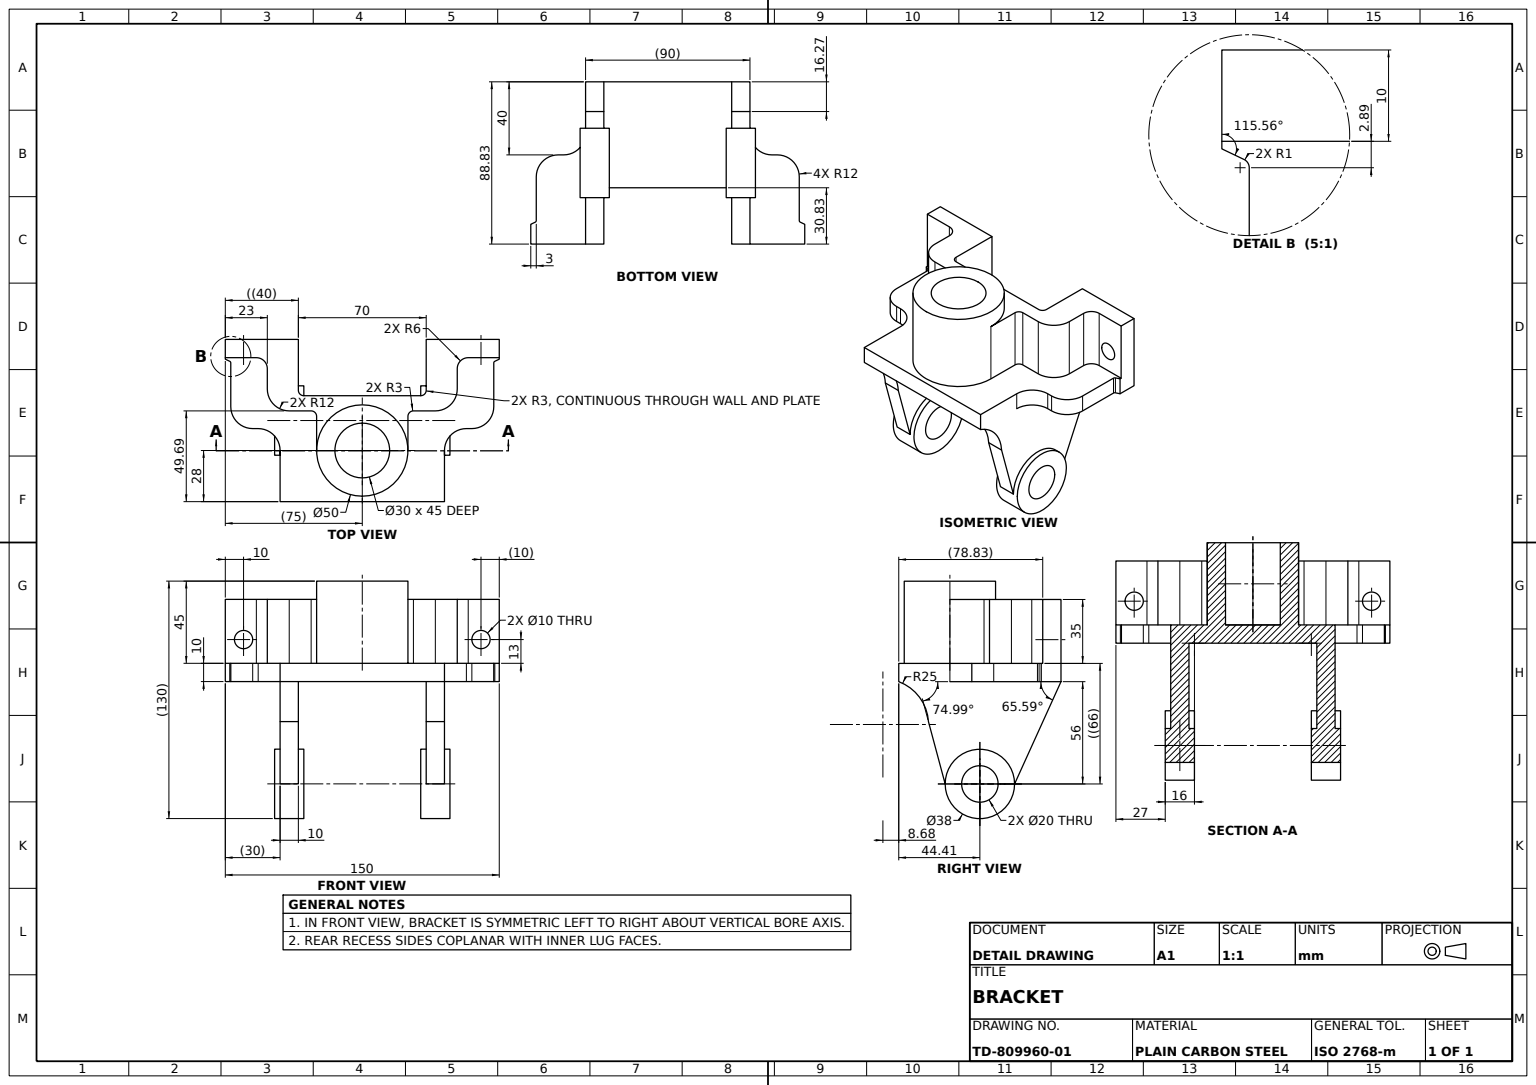
from build123d import *

# Parameters (mm, degrees)
BASE_PLATE_DEPTH        = 5
RISER_BLOCK_SKETCH_W    = 40
RISER_BLOCK_SKETCH_H    = 10.827146282
RISER_BLOCK_DEPTH       = 10
UPRIGHT_START           = 35
UPRIGHT_BOSS_35MM_DEPTH = 35
UPRIGHT_START_2         = 45
UPRIGHT_BOSS_45MM_DEPTH = 45
BORE_SKETCH_R           = 5
BORE_CUT_DEPTH          = 22.5
MOUNTING_LUG_DEPTH      = 10
LUG_BOSS_SKETCH_R       = 19
LUG_BOSS_SKETCH_R_2     = 10
LUG_BOSS_DEPTH          = 8


with BuildPart() as part:
    # Base Plate Sketch → Base Plate (new, symmetric)
    with BuildSketch(Plane(origin=(0, 0, 0), x_dir=(1, 0, 0), z_dir=(0, 1, 0))):
        with BuildLine():
            Line((-45, 0), (45, 0))
            Line((45, 0), (45, 28))
            ThreePointArc((45, 28), (48.514718626, 36.485281374), (57, 40))
            Line((57, 40), (60, 40))
            ThreePointArc((60, 40), (68.485281374, 43.514718626), (72, 52))
            Line((72, 52), (72, 75.935046753))
            ThreePointArc((72, 75.935046753), (72.153997607, 76.468225851), (72.568559901, 76.837188339))
            Line((72.568559901, 76.837188339), (75, 78))
            Line((75, 78), (72, 78))
            Line((72, 78), (35, 78))
            Line((35, 78), (35, 61))
            ThreePointArc((35, 61), (34.121320344, 58.878679656), (32, 58))
            Line((32, 58), (-32, 58))
            ThreePointArc((-32, 58), (-34.121320344, 58.878679656), (-35, 61))
            Line((-35, 61), (-35, 78))
            Line((-35, 78), (-72, 78))
            Line((-72, 78), (-75, 78))
            Line((-75, 78), (-72.568559901, 76.837188339))
            ThreePointArc((-72.568559901, 76.837188339), (-72.153997607, 76.468225851), (-72, 75.935046753))
            Line((-72, 75.935046753), (-72, 52))
            ThreePointArc((-72, 52), (-68.485281374, 43.514718626), (-60, 40))
            Line((-60, 40), (-57, 40))
            ThreePointArc((-57, 40), (-48.514718626, 36.485281374), (-45, 28))
            Line((-45, 28), (-45, 0))
        make_face()
    extrude(amount=BASE_PLATE_DEPTH, both=True)

    # Riser Block Sketch → Riser Block (add)
    with BuildSketch(Plane(origin=(0, 5, 0), x_dir=(1, 0, 0), z_dir=(0, 1, 0))):
        with Locations((-55, 83.413573141)):
            Rectangle(RISER_BLOCK_SKETCH_W, RISER_BLOCK_SKETCH_H)
        with Locations((55, 83.413573141)):
            Rectangle(RISER_BLOCK_SKETCH_W, RISER_BLOCK_SKETCH_H)
    extrude(amount=-RISER_BLOCK_DEPTH)

    # Upright Bosses Sketch → Upright Boss 35mm (add)
    with BuildSketch(Plane(origin=(0, 5, 0), x_dir=(1, 0, 0), z_dir=(0, 1, 0)).offset(UPRIGHT_START)):
        with BuildLine():
            Line((0, 53), (0, 58))
            Line((0, 58), (-32, 58))
            ThreePointArc((-32, 58), (-34.121320344, 58.878679656), (-35, 61))
            Line((-35, 61), (-35, 88.827146282))
            Line((-35, 88.827146282), (-75, 88.827146282))
            Line((-75, 88.827146282), (-75, 78.827146282))
            Line((-75, 78.827146282), (-58, 78.827146282))
            ThreePointArc((-58, 78.827146282), (-53.757359313, 77.069786969), (-52, 72.827146282))
            Line((-52, 72.827146282), (-52, 61.686127822))
            ThreePointArc((-52, 61.686127822), (-48.485281374, 53.200846447), (-40, 49.686127822))
            Line((-40, 49.686127822), (-28, 49.686127822))
            ThreePointArc((-28, 49.686127822), (-25.878679656, 48.807448165), (-25, 46.686127822))
            Line((-25, 46.686127822), (-25, 28))
            ThreePointArc((-25, 28), (-17.67766953, 45.67766953), (0, 53))
        make_face()
        with BuildLine():
            Line((75, 78.827146282), (75, 88.827146282))
            Line((75, 88.827146282), (35, 88.827146282))
            Line((35, 88.827146282), (35, 61))
            ThreePointArc((35, 61), (34.121320344, 58.878679656), (32, 58))
            Line((32, 58), (0, 58))
            Line((0, 58), (0, 53))
            ThreePointArc((0, 53), (17.67766953, 45.67766953), (25, 28))
            Line((25, 28), (25, 46.686127822))
            ThreePointArc((25, 46.686127822), (25.878679656, 48.807448165), (28, 49.686127822))
            Line((28, 49.686127822), (40, 49.686127822))
            ThreePointArc((40, 49.686127822), (48.485281374, 53.200846447), (52, 61.686127822))
            Line((52, 61.686127822), (52, 72.827146282))
            ThreePointArc((52, 72.827146282), (53.757359313, 77.069786969), (58, 78.827146282))
            Line((58, 78.827146282), (75, 78.827146282))
        make_face()
    extrude(amount=-UPRIGHT_BOSS_35MM_DEPTH)

    # Sketch5_3 → Upright Boss 45mm (add)
    with BuildSketch(Plane(origin=(0, 5, 0), x_dir=(1, 0, 0), z_dir=(0, 1, 0)).offset(UPRIGHT_START_2)):
        with BuildLine():
            ThreePointArc((25, 28), (17.67766953, 45.67766953), (0, 53))
            Line((0, 53), (0, 43))
            ThreePointArc((0, 43), (10.606601718, 38.606601718), (15, 28))
            ThreePointArc((15, 28), (10.606601718, 17.393398282), (0, 13))
            Line((0, 13), (0, 3))
            ThreePointArc((0, 3), (17.67766953, 10.32233047), (25, 28))
        make_face()
        with BuildLine():
            Line((0, 43), (0, 53))
            ThreePointArc((0, 53), (-17.67766953, 45.67766953), (-25, 28))
            ThreePointArc((-25, 28), (-17.67766953, 10.32233047), (0, 3))
            Line((0, 3), (0, 13))
            ThreePointArc((0, 13), (-15, 28), (0, 43))
        make_face()
        with BuildLine():
            ThreePointArc((25, 28), (17.67766953, 45.67766953), (0, 53))
            Line((0, 53), (0, 43))
            ThreePointArc((0, 43), (10.606601718, 38.606601718), (15, 28))
            ThreePointArc((15, 28), (10.606601718, 17.393398282), (0, 13))
            Line((0, 13), (0, 3))
            ThreePointArc((0, 3), (17.67766953, 10.32233047), (25, 28))
        make_face()
        with BuildLine():
            Line((0, 43), (0, 53))
            ThreePointArc((0, 53), (-17.67766953, 45.67766953), (-25, 28))
            ThreePointArc((-25, 28), (-17.67766953, 10.32233047), (0, 3))
            Line((0, 3), (0, 13))
            ThreePointArc((0, 13), (-15, 28), (0, 43))
        make_face()
    extrude(amount=-UPRIGHT_BOSS_45MM_DEPTH)

    # Bore Sketch → Bore Cut (cut, symmetric)
    with BuildSketch(Plane(origin=(0, 0, -88.827146282), x_dir=(-1, 0, 0), z_dir=(0, 0, -1))):
        with Locations((65, 18)):
            Circle(BORE_SKETCH_R)
        with Locations((-65, 18)):
            Circle(BORE_SKETCH_R)
    extrude(amount=BORE_CUT_DEPTH, both=True, mode=Mode.SUBTRACT)

    # Mounting Lug Sketch → Mounting Lug (add)
    with BuildSketch(Plane.ZY.offset(45)):
        with BuildLine():
            Line((-44.413573141, -5), (-88.827146282, -5))
            Line((-88.827146282, -5), (-63.413573141, -61))
            ThreePointArc((-63.413573141, -61), (-57.848601984, -47.564971157), (-44.413573141, -42))
            Line((-44.413573141, -42), (-44.413573141, -5))
        make_face()
        with BuildLine():
            Line((-28, -5), (-44.413573141, -5))
            Line((-44.413573141, -5), (-44.413573141, -42))
            ThreePointArc((-44.413573141, -42), (-30.978544299, -47.564971157), (-25.413573141, -61))
            Line((-25.413573141, -61), (-16.270280631, -26.90885398))
            ThreePointArc((-16.270280631, -26.90885398), (-11.388179119, -13.538606689), (0, -5))
            Line((0, -5), (-28, -5))
        make_face()
    mounting_lug = extrude(amount=-MOUNTING_LUG_DEPTH)

    # Lug Boss Sketch → Lug Boss (add, symmetric)
    with BuildSketch(Plane.ZY.offset(40)):
        with Locations((-44.413573141, -61)):
            Circle(LUG_BOSS_SKETCH_R)
        with Locations((-44.413573141, -61)):
            Circle(LUG_BOSS_SKETCH_R_2, mode=Mode.SUBTRACT)
    lug_boss = extrude(amount=LUG_BOSS_DEPTH, both=True)

    # Lug Mirror: Mounting Lug, Lug Boss across plane
    add(mounting_lug.mirror(Plane(origin=(0, 0, 0), x_dir=(0, 0, 1), z_dir=(1, 0, 0))))
    add(lug_boss.mirror(Plane(origin=(0, 0, 0), x_dir=(0, 0, 1), z_dir=(1, 0, 0))))


solid = part.part
